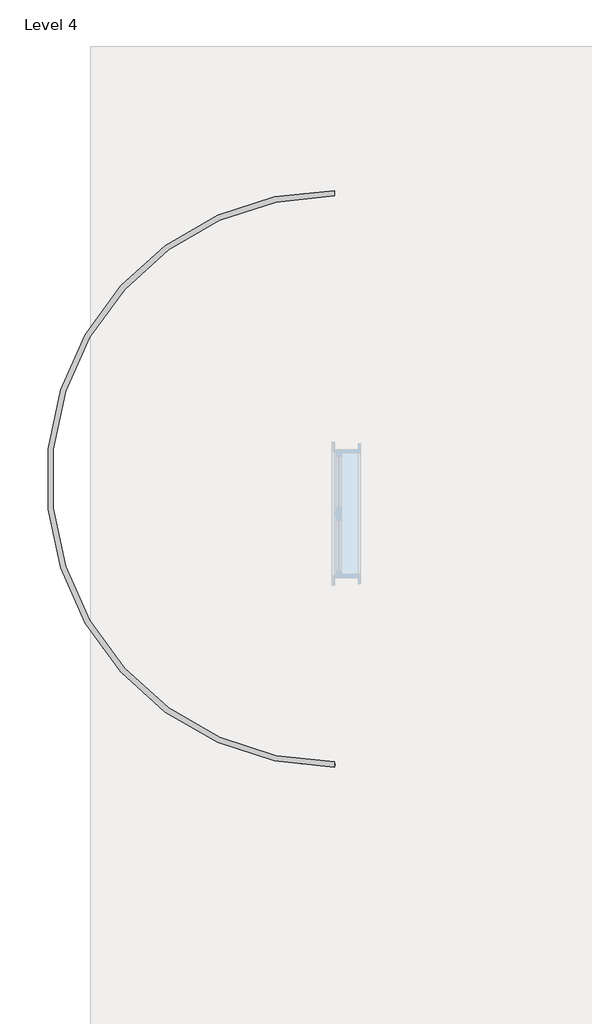
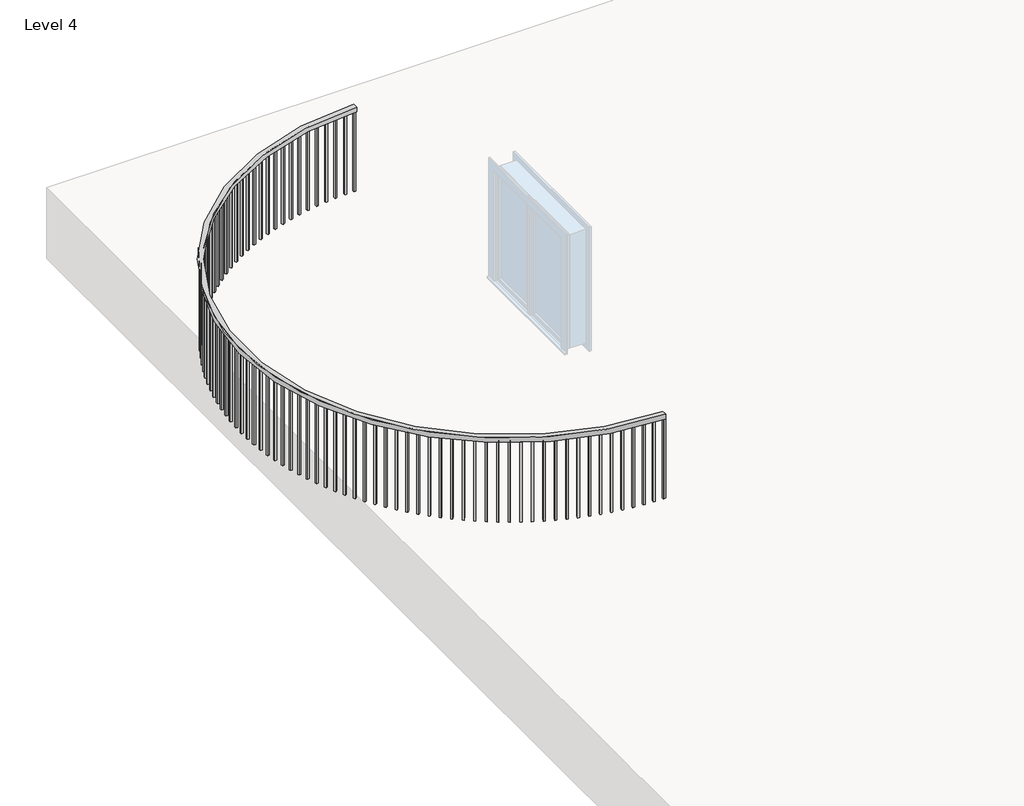
# One storey, part 2 of 2: 1 railing.
"""IFC4 building model written with IfcOpenShell, lengths in millimetres."""

from ifc_helpers import new_model, si_unit, point, frame, frame_2d, origin, place, context, project, spatial, polyline, circle_curve, trimmed, segment, composite_curve, outline, extrude, element, save

model = new_model("IFC4")

# Units and contexts
model_context = context("Model", 3, world=origin())
ifc_project = project(units=[si_unit("LENGTHUNIT", "METRE", prefix="MILLI")], contexts=[model_context])

# Site, building, storey
site = spatial("IfcSite", under=ifc_project)
building = spatial("IfcBuilding", under=site)
storey = spatial("IfcBuildingStorey", under=building, Name="Level 4", Elevation=9144.0)

# Railing
placement = place(None, origin())
element("IfcRailing", 1, ObjectType="Handrail - Rectangular", at=placement, inside=storey, context=model_context, shape_type="SweptSolid", body=[
    extrude(outline(composite_curve([segment(trimmed(circle_curve(frame_2d((-15728.6368919, 10326.9945075)), 2743.2), [point((-15728.6368919, 7583.7945075))], [point((-15728.6368919, 13070.1945075))], False, "CARTESIAN"), True, "CONTINUOUS"), segment(polyline([(-15728.6368919, 13070.1945075), (-15728.6368919, 13019.3945075)]), True, "CONTINUOUS"), segment(trimmed(circle_curve(frame_2d((-15728.6368919, 10326.9945075)), 2692.4), [point((-15728.6368919, 13019.3945075))], [point((-15728.6368919, 7634.5945075))], True, "CARTESIAN"), True, "CONTINUOUS"), segment(polyline([(-15728.6368919, 7634.5945075), (-15728.6368919, 7583.7945075)]), True, "CONTINUOUS")], self_intersect=False)), frame((0.0, 0.0, 10007.6), z_axis=(0.0, 0.0, 1.0), x_axis=(1.0, 0.0, 0.0)), (0.0, 0.0, 1.0), 50.8),
    extrude(outline(polyline([(-15741.9957848, 7599.6855919), (-15741.9690055, 7618.735573), (-15722.9190243, 7618.7087937), (-15722.9458036, 7599.6588126), (-15741.9957848, 7599.6855919)])), frame((0.0, 0.0, 9144.0), z_axis=(0.0, 0.0, 1.0), x_axis=(1.0, 0.0, 0.0)), (0.0, 0.0, 1.0), 863.6),
    extrude(outline(polyline([(-15843.9181793, 7602.0903613), (-15843.1794358, 7621.1260319), (-15824.1437651, 7620.3872884), (-15824.8825087, 7601.3516177), (-15843.9181793, 7602.0903613)])), frame((0.0, 0.0, 9144.0), z_axis=(0.0, 0.0, 1.0), x_axis=(1.0, 0.0, 0.0)), (0.0, 0.0, 1.0), 863.6),
    extrude(outline(polyline([(-15945.6794868, 7608.3027461), (-15944.2298113, 7627.297507), (-15925.2350504, 7625.8478315), (-15926.6847259, 7606.8530706), (-15945.6794868, 7608.3027461)])), frame((0.0, 0.0, 9144.0), z_axis=(0.0, 0.0, 1.0), x_axis=(1.0, 0.0, 0.0)), (0.0, 0.0, 1.0), 863.6),
    extrude(outline(polyline([(-16047.1375121, 7618.3140656), (-16044.9789303, 7637.2413746), (-16026.0516213, 7635.0827927), (-16028.2102032, 7616.1554838), (-16047.1375121, 7618.3140656)])), frame((0.0, 0.0, 9144.0), z_axis=(0.0, 0.0, 1.0), x_axis=(1.0, 0.0, 0.0)), (0.0, 0.0, 1.0), 863.6),
    extrude(outline(polyline([(-16148.150484, 7632.1103305), (-16145.2860122, 7650.9437397), (-16126.452603, 7648.0792678), (-16129.3170749, 7629.2458587), (-16148.150484, 7632.1103305)])), frame((0.0, 0.0, 9144.0), z_axis=(0.0, 0.0, 1.0), x_axis=(1.0, 0.0, 0.0)), (0.0, 0.0, 1.0), 863.6),
    extrude(outline(polyline([(-16248.5772532, 7649.6722628), (-16245.0108939, 7668.3854555), (-16226.2977012, 7664.8190963), (-16229.8640605, 7646.1059035), (-16248.5772532, 7649.6722628)])), frame((0.0, 0.0, 9144.0), z_axis=(0.0, 0.0, 1.0), x_axis=(1.0, 0.0, 0.0)), (0.0, 0.0, 1.0), 863.6),
    extrude(outline(polyline([(-16348.2774892, 7670.9753224), (-16344.014226, 7689.54215), (-16325.4473984, 7685.2788868), (-16329.7106616, 7666.7120592), (-16348.2774892, 7670.9753224)])), frame((0.0, 0.0, 9144.0), z_axis=(0.0, 0.0, 1.0), x_axis=(1.0, 0.0, 0.0)), (0.0, 0.0, 1.0), 863.6),
    extrude(outline(polyline([(-16447.1118772, 7695.9897418), (-16442.1576672, 7714.3842602), (-16423.7631489, 7709.4300502), (-16428.7173589, 7691.0355319), (-16447.1118772, 7695.9897418)])), frame((0.0, 0.0, 9144.0), z_axis=(0.0, 0.0, 1.0), x_axis=(1.0, 0.0, 0.0)), (0.0, 0.0, 1.0), 863.6),
    extrude(outline(polyline([(-16544.9423119, 7724.6805674), (-16539.3040779, 7742.8770731), (-16521.1075722, 7737.2388391), (-16526.7458062, 7719.0423334), (-16544.9423119, 7724.6805674)])), frame((0.0, 0.0, 9144.0), z_axis=(0.0, 0.0, 1.0), x_axis=(1.0, 0.0, 0.0)), (0.0, 0.0, 1.0), 863.6),
    extrude(outline(polyline([(-16641.632091, 7757.0077083), (-16635.3177115, 7774.9807746), (-16617.3446452, 7768.6663951), (-16623.6590247, 7750.6933288), (-16641.632091, 7757.0077083)])), frame((0.0, 0.0, 9144.0), z_axis=(0.0, 0.0, 1.0), x_axis=(1.0, 0.0, 0.0)), (0.0, 0.0, 1.0), 863.6),
    extrude(outline(polyline([(-16737.0461061, 7792.9259926), (-16730.0644044, 7810.6505051), (-16712.3398919, 7803.6688034), (-16719.3215936, 7785.9442909), (-16737.0461061, 7792.9259926)])), frame((0.0, 0.0, 9144.0), z_axis=(0.0, 0.0, 1.0), x_axis=(1.0, 0.0, 0.0)), (0.0, 0.0, 1.0), 863.6),
    extrude(outline(polyline([(-16831.0510314, 7832.3852302), (-16823.4117634, 7849.8364217), (-16805.9605719, 7842.1971536), (-16813.59984, 7824.7459621), (-16831.0510314, 7832.3852302)])), frame((0.0, 0.0, 9144.0), z_axis=(0.0, 0.0, 1.0), x_axis=(1.0, 0.0, 0.0)), (0.0, 0.0, 1.0), 863.6),
    extrude(outline(polyline([(-16923.5155103, 7875.3302832), (-16915.2293505, 7892.4837684), (-16898.0758652, 7884.1976086), (-16906.362025, 7867.0441234), (-16923.5155103, 7875.3302832)])), frame((0.0, 0.0, 9144.0), z_axis=(0.0, 0.0, 1.0), x_axis=(1.0, 0.0, 0.0)), (0.0, 0.0, 1.0), 863.6),
    extrude(outline(polyline([(-17014.3103383, 7921.7011427), (-17005.3888654, 7938.5329525), (-16988.5570556, 7929.6114796), (-16997.4785285, 7912.7796698), (-17014.3103383, 7921.7011427)])), frame((0.0, 0.0, 9144.0), z_axis=(0.0, 0.0, 1.0), x_axis=(1.0, 0.0, 0.0)), (0.0, 0.0, 1.0), 863.6),
    extrude(outline(polyline([(-17103.3086445, 7971.4330131), (-17093.7643247, 7987.9196276), (-17077.2777101, 7978.3753079), (-17086.8220299, 7961.8886933), (-17103.3086445, 7971.4330131)])), frame((0.0, 0.0, 9144.0), z_axis=(0.0, 0.0, 1.0), x_axis=(1.0, 0.0, 0.0)), (0.0, 0.0, 1.0), 863.6),
    extrude(outline(polyline([(-17190.3860679, 8024.4564019), (-17180.2322379, 8040.5747838), (-17164.1138559, 8030.4209539), (-17174.2676859, 8014.3025719), (-17190.3860679, 8024.4564019)])), frame((0.0, 0.0, 9144.0), z_axis=(0.0, 0.0, 1.0), x_axis=(1.0, 0.0, 0.0)), (0.0, 0.0, 1.0), 863.6),
    extrude(outline(polyline([(-17275.4209318, 8080.6972174), (-17264.67178, 8096.424844), (-17248.9441535, 8085.6756922), (-17259.6933053, 8069.9480657), (-17275.4209318, 8080.6972174)])), frame((0.0, 0.0, 9144.0), z_axis=(0.0, 0.0, 1.0), x_axis=(1.0, 0.0, 0.0)), (0.0, 0.0, 1.0), 863.6),
    extrude(outline(polyline([(-17358.2944137, 8140.0768723), (-17346.9649603, 8155.3917666), (-17331.6500661, 8144.0623132), (-17342.9795194, 8128.747419), (-17358.2944137, 8140.0768723)])), frame((0.0, 0.0, 9144.0), z_axis=(0.0, 0.0, 1.0), x_axis=(1.0, 0.0, 0.0)), (0.0, 0.0, 1.0), 863.6),
    extrude(outline(polyline([(-17438.8907113, 8202.512393), (-17426.9967874, 8217.3931549), (-17412.1160255, 8205.499231), (-17424.0099494, 8190.6184691), (-17438.8907113, 8202.512393)])), frame((0.0, 0.0, 9144.0), z_axis=(0.0, 0.0, 1.0), x_axis=(1.0, 0.0, 0.0)), (0.0, 0.0, 1.0), 863.6),
    extrude(outline(polyline([(-17517.0972041, 8267.9165359), (-17504.6554295, 8282.3423719), (-17490.2295935, 8269.9005973), (-17502.671368, 8255.4747613), (-17517.0972041, 8267.9165359)])), frame((0.0, 0.0, 9144.0), z_axis=(0.0, 0.0, 1.0), x_axis=(1.0, 0.0, 0.0)), (0.0, 0.0, 1.0), 863.6),
    extrude(outline(polyline([(-17592.8046111, 8336.1979092), (-17579.8323713, 8350.1486616), (-17565.8816189, 8337.1764217), (-17578.8538587, 8323.2256693), (-17592.8046111, 8336.1979092)])), frame((0.0, 0.0, 9144.0), z_axis=(0.0, 0.0, 1.0), x_axis=(1.0, 0.0, 0.0)), (0.0, 0.0, 1.0), 863.6),
    extrude(outline(polyline([(-17665.9071435, 8407.2611006), (-17652.422565, 8420.7172754), (-17638.9663901, 8407.2326969), (-17652.4509687, 8393.7765221), (-17665.9071435, 8407.2611006)])), frame((0.0, 0.0, 9144.0), z_axis=(0.0, 0.0, 1.0), x_axis=(1.0, 0.0, 0.0)), (0.0, 0.0, 1.0), 863.6),
    extrude(outline(polyline([(-17736.3026522, 8481.0068109), (-17722.3245775, 8493.9496053), (-17709.3817831, 8479.9715306), (-17723.3598578, 8467.0287361), (-17736.3026522, 8481.0068109)])), frame((0.0, 0.0, 9144.0), z_axis=(0.0, 0.0, 1.0), x_axis=(1.0, 0.0, 0.0)), (0.0, 0.0, 1.0), 863.6),
    extrude(outline(polyline([(-17803.8927708, 8557.3319921), (-17789.4407321, 8569.7433206), (-17777.0294035, 8555.2912819), (-17791.4814423, 8542.8799533), (-17803.8927708, 8557.3319921)])), frame((0.0, 0.0, 9144.0), z_axis=(0.0, 0.0, 1.0), x_axis=(1.0, 0.0, 0.0)), (0.0, 0.0, 1.0), 863.6),
    extrude(outline(polyline([(-17868.583053, 8636.1299922), (-17853.6772446, 8647.992512), (-17841.8147248, 8633.0867036), (-17856.7205331, 8621.2241838), (-17868.583053, 8636.1299922)])), frame((0.0, 0.0, 9144.0), z_axis=(0.0, 0.0, 1.0), x_axis=(1.0, 0.0, 0.0)), (0.0, 0.0, 1.0), 863.6),
    extrude(outline(polyline([(-17930.2831044, 8717.2907036), (-17914.9443548, 8728.5878387), (-17903.6472197, 8713.2490891), (-17918.9859693, 8701.951954), (-17930.2831044, 8717.2907036)])), frame((0.0, 0.0, 9144.0), z_axis=(0.0, 0.0, 1.0), x_axis=(1.0, 0.0, 0.0)), (0.0, 0.0, 1.0), 863.6),
    extrude(outline(polyline([(-17988.9067092, 8800.7007172), (-17973.1564519, 8811.4166817), (-17962.4404874, 8795.6664245), (-17978.1907447, 8784.9504599), (-17988.9067092, 8800.7007172)])), frame((0.0, 0.0, 9144.0), z_axis=(0.0, 0.0, 1.0), x_axis=(1.0, 0.0, 0.0)), (0.0, 0.0, 1.0), 863.6),
    extrude(outline(polyline([(-18044.3719504, 8886.2434811), (-18028.2321938, 8896.3633011), (-18018.1123738, 8880.2235446), (-18034.2521303, 8870.1037245), (-18044.3719504, 8886.2434811)])), frame((0.0, 0.0, 9144.0), z_axis=(0.0, 0.0, 1.0), x_axis=(1.0, 0.0, 0.0)), (0.0, 0.0, 1.0), 863.6),
    extrude(outline(polyline([(-18096.6013241, 8973.7994628), (-18080.094621, 8983.3089976), (-18070.5850862, 8966.8022945), (-18087.0917894, 8957.2927597), (-18096.6013241, 8973.7994628)])), frame((0.0, 0.0, 9144.0), z_axis=(0.0, 0.0, 1.0), x_axis=(1.0, 0.0, 0.0)), (0.0, 0.0, 1.0), 863.6),
    extrude(outline(polyline([(-18145.5218483, 9063.2463171), (-18128.6712641, 9072.1322785), (-18119.7853026, 9055.2816943), (-18136.6358868, 9046.3957328), (-18145.5218483, 9063.2463171)])), frame((0.0, 0.0, 9144.0), z_axis=(0.0, 0.0, 1.0), x_axis=(1.0, 0.0, 0.0)), (0.0, 0.0, 1.0), 863.6),
    extrude(outline(polyline([(-18191.0651643, 9154.4590562), (-18173.894245, 9162.7090277), (-18165.6442735, 9145.5381083), (-18182.8151929, 9137.2881369), (-18191.0651643, 9154.4590562)])), frame((0.0, 0.0, 9144.0), z_axis=(0.0, 0.0, 1.0), x_axis=(1.0, 0.0, 0.0)), (0.0, 0.0, 1.0), 863.6),
    extrude(outline(polyline([(-18233.1676328, 9247.3102252), (-18215.7003719, 9254.9126786), (-18208.0979185, 9237.4454177), (-18225.5651793, 9229.8429643), (-18233.1676328, 9247.3102252)])), frame((0.0, 0.0, 9144.0), z_axis=(0.0, 0.0, 1.0), x_axis=(1.0, 0.0, 0.0)), (0.0, 0.0, 1.0), 863.6),
    extrude(outline(polyline([(-18271.7704221, 9341.6700793), (-18254.0312274, 9348.6143915), (-18247.0869153, 9330.8751968), (-18264.82611, 9323.9308846), (-18271.7704221, 9341.6700793)])), frame((0.0, 0.0, 9144.0), z_axis=(0.0, 0.0, 1.0), x_axis=(1.0, 0.0, 0.0)), (0.0, 0.0, 1.0), 863.6),
    extrude(outline(polyline([(-18306.8195913, 9437.4067659), (-18288.8332504, 9443.6832333), (-18282.5567831, 9425.6968925), (-18300.5431239, 9419.4204251), (-18306.8195913, 9437.4067659)])), frame((0.0, 0.0, 9144.0), z_axis=(0.0, 0.0, 1.0), x_axis=(1.0, 0.0, 0.0)), (0.0, 0.0, 1.0), 863.6),
    extrude(outline(polyline([(-18338.2661646, 9534.3865084), (-18320.0578106, 9539.9863606), (-18314.4579584, 9521.7780066), (-18332.6663124, 9516.1781544), (-18338.2661646, 9534.3865084)])), frame((0.0, 0.0, 9144.0), z_axis=(0.0, 0.0, 1.0), x_axis=(1.0, 0.0, 0.0)), (0.0, 0.0, 1.0), 863.6),
    extrude(outline(polyline([(-18366.0662006, 9632.4737931), (-18347.6612768, 9637.3892053), (-18342.7458646, 9618.9842814), (-18361.1507885, 9614.0688692), (-18366.0662006, 9632.4737931)])), frame((0.0, 0.0, 9144.0), z_axis=(0.0, 0.0, 1.0), x_axis=(1.0, 0.0, 0.0)), (0.0, 0.0, 1.0), 863.6),
    extrude(outline(polyline([(-18390.1808532, 9731.5315588), (-18371.6050774, 9735.7556625), (-18367.3809737, 9717.1798866), (-18385.9567496, 9712.955783), (-18390.1808532, 9731.5315588)])), frame((0.0, 0.0, 9144.0), z_axis=(0.0, 0.0, 1.0), x_axis=(1.0, 0.0, 0.0)), (0.0, 0.0, 1.0), 863.6),
    extrude(outline(polyline([(-18410.576426, 9831.4213883), (-18391.8557549, 9834.9482809), (-18388.3288623, 9816.2276097), (-18407.0495335, 9812.7007171), (-18410.576426, 9831.4213883)])), frame((0.0, 0.0, 9144.0), z_axis=(0.0, 0.0, 1.0), x_axis=(1.0, 0.0, 0.0)), (0.0, 0.0, 1.0), 863.6),
    extrude(outline(polyline([(-18427.2244196, 9932.0037015), (-18408.3850122, 9934.8284548), (-18405.560259, 9915.9890475), (-18424.3996663, 9913.1642942), (-18427.2244196, 9932.0037015)])), frame((0.0, 0.0, 9144.0), z_axis=(0.0, 0.0, 1.0), x_axis=(1.0, 0.0, 0.0)), (0.0, 0.0, 1.0), 863.6),
    extrude(outline(polyline([(-18440.1015709, 10033.1379509), (-18421.1697524, 10035.2566177), (-18419.0510856, 10016.3247992), (-18437.9829041, 10014.2061324), (-18440.1015709, 10033.1379509)])), frame((0.0, 0.0, 9144.0), z_axis=(0.0, 0.0, 1.0), x_axis=(1.0, 0.0, 0.0)), (0.0, 0.0, 1.0), 863.6),
    extrude(outline(polyline([(-18449.1898863, 10134.6828176), (-18430.1921108, 10136.0924374), (-18428.782491, 10117.094662), (-18447.7802664, 10115.6850421), (-18449.1898863, 10134.6828176)])), frame((0.0, 0.0, 9144.0), z_axis=(0.0, 0.0, 1.0), x_axis=(1.0, 0.0, 0.0)), (0.0, 0.0, 1.0), 863.6),
    extrude(outline(polyline([(-18454.4766663, 10236.4964089), (-18435.4394802, 10237.1950121), (-18434.740877, 10218.157826), (-18453.7780631, 10217.4592228), (-18454.4766663, 10236.4964089)])), frame((0.0, 0.0, 9144.0), z_axis=(0.0, 0.0, 1.0), x_axis=(1.0, 0.0, 0.0)), (0.0, 0.0, 1.0), 863.6),
    extrude(outline(polyline([(-18455.9545234, 10338.4364568), (-18436.9045281, 10338.4230671), (-18436.9179178, 10319.3730718), (-18455.967913, 10319.3864615), (-18455.9545234, 10338.4364568)])), frame((0.0, 0.0, 9144.0), z_axis=(0.0, 0.0, 1.0), x_axis=(1.0, 0.0, 0.0)), (0.0, 0.0, 1.0), 863.6),
    extrude(outline(polyline([(-18453.6213926, 10440.3605163), (-18434.5852074, 10439.6351526), (-18435.3105712, 10420.5989673), (-18454.3467564, 10421.3243311), (-18453.6213926, 10440.3605163)])), frame((0.0, 0.0, 9144.0), z_axis=(0.0, 0.0, 1.0), x_axis=(1.0, 0.0, 0.0)), (0.0, 0.0, 1.0), 863.6),
    extrude(outline(polyline([(-18447.4805342, 10542.1261652), (-18428.4847591, 10540.6898408), (-18429.9210834, 10521.6940657), (-18448.9168585, 10523.13039), (-18447.4805342, 10542.1261652)])), frame((0.0, 0.0, 9144.0), z_axis=(0.0, 0.0, 1.0), x_axis=(1.0, 0.0, 0.0)), (0.0, 0.0, 1.0), 863.6),
    extrude(outline(polyline([(-18437.5405288, 10643.5912021), (-18418.6117074, 10641.4459242), (-18420.7569852, 10622.5171027), (-18439.6858067, 10624.6623806), (-18437.5405288, 10643.5912021)])), frame((0.0, 0.0, 9144.0), z_axis=(0.0, 0.0, 1.0), x_axis=(1.0, 0.0, 0.0)), (0.0, 0.0, 1.0), 863.6),
    extrude(outline(polyline([(-18423.8152662, 10744.613846), (-18404.9798483, 10741.7626123), (-18407.8310821, 10722.9271944), (-18426.6664999, 10725.7784281), (-18423.8152662, 10744.613846)])), frame((0.0, 0.0, 9144.0), z_axis=(0.0, 0.0, 1.0), x_axis=(1.0, 0.0, 0.0)), (0.0, 0.0, 1.0), 863.6),
    extrude(outline(polyline([(-18406.3239251, 10845.0529341), (-18387.6082304, 10841.4997286), (-18391.1614358, 10822.7840338), (-18409.8771306, 10826.3372393), (-18406.3239251, 10845.0529341)])), frame((0.0, 0.0, 9144.0), z_axis=(0.0, 0.0, 1.0), x_axis=(1.0, 0.0, 0.0)), (0.0, 0.0, 1.0), 863.6),
    extrude(outline(polyline([(-18385.0909469, 10944.7681188), (-18366.5211274, 10940.5179066), (-18370.7713395, 10921.9480871), (-18389.341159, 10926.1982992), (-18385.0909469, 10944.7681188)])), frame((0.0, 0.0, 9144.0), z_axis=(0.0, 0.0, 1.0), x_axis=(1.0, 0.0, 0.0)), (0.0, 0.0, 1.0), 863.6),
    extrude(outline(polyline([(-18360.1460013, 11043.6200641), (-18341.7480054, 11038.6787843), (-18346.6892852, 11020.2807884), (-18365.0872811, 11025.2220682), (-18360.1460013, 11043.6200641)])), frame((0.0, 0.0, 9144.0), z_axis=(0.0, 0.0, 1.0), x_axis=(1.0, 0.0, 0.0)), (0.0, 0.0, 1.0), 863.6),
    extrude(outline(polyline([(-18331.5239448, 11141.4706405), (-18313.3234807, 11135.8451977), (-18318.9489235, 11117.6447336), (-18337.1493876, 11123.2701765), (-18331.5239448, 11141.4706405)])), frame((0.0, 0.0, 9144.0), z_axis=(0.0, 0.0, 1.0), x_axis=(1.0, 0.0, 0.0)), (0.0, 0.0, 1.0), 863.6),
    extrude(outline(polyline([(-18299.2647721, 11238.1831175), (-18281.287272, 11231.8813723), (-18287.5890173, 11213.9038722), (-18305.5665173, 11220.2056175), (-18299.2647721, 11238.1831175)])), frame((0.0, 0.0, 9144.0), z_axis=(0.0, 0.0, 1.0), x_axis=(1.0, 0.0, 0.0)), (0.0, 0.0, 1.0), 863.6),
    extrude(outline(polyline([(-18263.4135602, 11333.6223549), (-18245.6841449, 11326.6531129), (-18252.6533869, 11308.9236976), (-18270.3828021, 11315.8929396), (-18263.4135602, 11333.6223549)])), frame((0.0, 0.0, 9144.0), z_axis=(0.0, 0.0, 1.0), x_axis=(1.0, 0.0, 0.0)), (0.0, 0.0, 1.0), 863.6),
    extrude(outline(polyline([(-18224.0204055, 11427.6549917), (-18206.5638489, 11420.0279914), (-18214.1908492, 11402.5714348), (-18231.6474057, 11410.1984351), (-18224.0204055, 11427.6549917)])), frame((0.0, 0.0, 9144.0), z_axis=(0.0, 0.0, 1.0), x_axis=(1.0, 0.0, 0.0)), (0.0, 0.0, 1.0), 863.6),
    extrude(outline(polyline([(-18181.1403535, 11520.1496324), (-18163.9810484, 11511.8755313), (-18172.2551495, 11494.7162262), (-18189.4144546, 11502.9903273), (-18181.1403535, 11520.1496324)])), frame((0.0, 0.0, 9144.0), z_axis=(0.0, 0.0, 1.0), x_axis=(1.0, 0.0, 0.0)), (0.0, 0.0, 1.0), 863.6),
    extrude(outline(polyline([(-18134.8333222, 11610.9770307), (-18117.995246, 11602.0673905), (-18126.9048862, 11585.2293142), (-18143.7429624, 11594.1389544), (-18134.8333222, 11610.9770307)])), frame((0.0, 0.0, 9144.0), z_axis=(0.0, 0.0, 1.0), x_axis=(1.0, 0.0, 0.0)), (0.0, 0.0, 1.0), 863.6),
    extrude(outline(polyline([(-18085.1640183, 11700.0102698), (-18068.6706994, 11690.4775403), (-18078.2034289, 11673.9842214), (-18094.6967478, 11683.5169509), (-18085.1640183, 11700.0102698)])), frame((0.0, 0.0, 9144.0), z_axis=(0.0, 0.0, 1.0), x_axis=(1.0, 0.0, 0.0)), (0.0, 0.0, 1.0), 863.6),
    extrude(outline(polyline([(-18032.2018467, 11787.1249402), (-18016.0763318, 11776.9824419), (-18026.2188302, 11760.8569271), (-18042.344345, 11770.9994254), (-18032.2018467, 11787.1249402)])), frame((0.0, 0.0, 9144.0), z_axis=(0.0, 0.0, 1.0), x_axis=(1.0, 0.0, 0.0)), (0.0, 0.0, 1.0), 863.6),
    extrude(outline(polyline([(-17976.0208133, 11872.199313), (-17960.2856354, 11861.4612184), (-17971.0237301, 11845.7260405), (-17986.758908, 11856.4641351), (-17976.0208133, 11872.199313)])), frame((0.0, 0.0, 9144.0), z_axis=(0.0, 0.0, 1.0), x_axis=(1.0, 0.0, 0.0)), (0.0, 0.0, 1.0), 863.6),
    extrude(outline(polyline([(-17916.6994223, 11955.1145106), (-17901.3765687, 11943.7958244), (-17912.6952549, 11928.4729708), (-17928.0181085, 11939.791657), (-17916.6994223, 11955.1145106)])), frame((0.0, 0.0, 9144.0), z_axis=(0.0, 0.0, 1.0), x_axis=(1.0, 0.0, 0.0)), (0.0, 0.0, 1.0), 863.6),
    extrude(outline(polyline([(-17854.3205656, 12035.7546722), (-17839.4314475, 12023.8712105), (-17851.3149093, 12008.9820924), (-17866.2040274, 12020.8655541), (-17854.3205656, 12035.7546722)])), frame((0.0, 0.0, 9144.0), z_axis=(0.0, 0.0, 1.0), x_axis=(1.0, 0.0, 0.0)), (0.0, 0.0, 1.0), 863.6),
    extrude(outline(polyline([(-17788.9714078, 12114.0071162), (-17774.5368304, 12101.5754842), (-17786.9684624, 12087.1409068), (-17801.4030399, 12099.5725388), (-17788.9714078, 12114.0071162)])), frame((0.0, 0.0, 9144.0), z_axis=(0.0, 0.0, 1.0), x_axis=(1.0, 0.0, 0.0)), (0.0, 0.0, 1.0), 863.6),
    extrude(outline(polyline([(-17720.7432638, 12189.7624974), (-17706.783397, 12176.8000663), (-17719.7458282, 12162.8401996), (-17733.7056949, 12175.8026307), (-17720.7432638, 12189.7624974)])), frame((0.0, 0.0, 9144.0), z_axis=(0.0, 0.0, 1.0), x_axis=(1.0, 0.0, 0.0)), (0.0, 0.0, 1.0), 863.6),
    extrude(outline(polyline([(-17649.7314714, 12262.9149599), (-17636.265822, 12249.4398426), (-17649.7409393, 12235.9741932), (-17663.2065887, 12249.4493105), (-17649.7314714, 12262.9149599)])), frame((0.0, 0.0, 9144.0), z_axis=(0.0, 0.0, 1.0), x_axis=(1.0, 0.0, 0.0)), (0.0, 0.0, 1.0), 863.6),
    extrude(outline(polyline([(-17576.0352582, 12333.3622847), (-17563.0826422, 12319.3933106), (-17577.0516164, 12306.4406946), (-17590.0042323, 12320.4096688), (-17576.0352582, 12333.3622847)])), frame((0.0, 0.0, 9144.0), z_axis=(0.0, 0.0, 1.0), x_axis=(1.0, 0.0, 0.0)), (0.0, 0.0, 1.0), 863.6),
    extrude(outline(polyline([(-17499.7576028, 12401.0060332), (-17487.3361194, 12386.5627216), (-17501.779431, 12374.1412382), (-17514.2009144, 12388.5845499), (-17499.7576028, 12401.0060332)])), frame((0.0, 0.0, 9144.0), z_axis=(0.0, 0.0, 1.0), x_axis=(1.0, 0.0, 0.0)), (0.0, 0.0, 1.0), 863.6),
    extrude(outline(polyline([(-17421.0050909, 12465.751684), (-17409.1320972, 12450.8542171), (-17424.0295641, 12438.9812234), (-17435.9025578, 12453.8786903), (-17421.0050909, 12465.751684)])), frame((0.0, 0.0, 9144.0), z_axis=(0.0, 0.0, 1.0), x_axis=(1.0, 0.0, 0.0)), (0.0, 0.0, 1.0), 863.6),
    extrude(outline(polyline([(-17339.8877666, 12527.5087656), (-17328.5798531, 12512.1779602), (-17343.9106585, 12500.8700467), (-17355.218572, 12516.2008521), (-17339.8877666, 12527.5087656)])), frame((0.0, 0.0, 9144.0), z_axis=(0.0, 0.0, 1.0), x_axis=(1.0, 0.0, 0.0)), (0.0, 0.0, 1.0), 863.6),
    extrude(outline(polyline([(-17256.5189783, 12586.1909822), (-17245.791946, 12570.4482607), (-17261.5346675, 12559.7212285), (-17272.2616997, 12575.46395), (-17256.5189783, 12586.1909822)])), frame((0.0, 0.0, 9144.0), z_axis=(0.0, 0.0, 1.0), x_axis=(1.0, 0.0, 0.0)), (0.0, 0.0, 1.0), 863.6),
    extrude(outline(polyline([(-17171.0152203, 12641.716335), (-17160.8840587, 12625.5836953), (-17177.0166983, 12615.4525337), (-17187.14786, 12631.5851733), (-17171.0152203, 12641.716335)])), frame((0.0, 0.0, 9144.0), z_axis=(0.0, 0.0, 1.0), x_axis=(1.0, 0.0, 0.0)), (0.0, 0.0, 1.0), 863.6),
    extrude(outline(polyline([(-17083.4959706, 12694.0072362), (-17073.9748361, 12677.5072211), (-17090.4748512, 12667.9860867), (-17099.9959857, 12684.4861018), (-17083.4959706, 12694.0072362)])), frame((0.0, 0.0, 9144.0), z_axis=(0.0, 0.0, 1.0), x_axis=(1.0, 0.0, 0.0)), (0.0, 0.0, 1.0), 863.6),
    extrude(outline(polyline([(-16994.0835232, 12742.9906177), (-16985.1857201, 12726.1462833), (-17002.0300546, 12717.2484803), (-17010.9278576, 12734.0928147), (-16994.0835232, 12742.9906177)])), frame((0.0, 0.0, 9144.0), z_axis=(0.0, 0.0, 1.0), x_axis=(1.0, 0.0, 0.0)), (0.0, 0.0, 1.0), 863.6),
    extrude(outline(polyline([(-16902.9028175, 12788.5980331), (-16894.6407792, 12771.4329166), (-16911.8058957, 12763.1708783), (-16920.067934, 12780.3359948), (-16902.9028175, 12788.5980331)])), frame((0.0, 0.0, 9144.0), z_axis=(0.0, 0.0, 1.0), x_axis=(1.0, 0.0, 0.0)), (0.0, 0.0, 1.0), 863.6),
    extrude(outline(polyline([(-16810.081264, 12830.7657533), (-16802.4665353, 12813.3038403), (-16819.9284483, 12805.6891115), (-16827.543177, 12823.1510246), (-16810.081264, 12830.7657533)])), frame((0.0, 0.0, 9144.0), z_axis=(0.0, 0.0, 1.0), x_axis=(1.0, 0.0, 0.0)), (0.0, 0.0, 1.0), 863.6),
    extrude(outline(polyline([(-16715.7485659, 12869.4348557), (-16708.7917871, 12851.7005464), (-16726.5260965, 12844.7437676), (-16733.4828752, 12862.4780769), (-16715.7485659, 12869.4348557)])), frame((0.0, 0.0, 9144.0), z_axis=(0.0, 0.0, 1.0), x_axis=(1.0, 0.0, 0.0)), (0.0, 0.0, 1.0), 863.6),
    extrude(outline(polyline([(-16620.0365379, 12904.5513065), (-16613.74743, 12886.5693817), (-16631.7293549, 12880.2802738), (-16638.0184627, 12898.2621987), (-16620.0365379, 12904.5513065)])), frame((0.0, 0.0, 9144.0), z_axis=(0.0, 0.0, 1.0), x_axis=(1.0, 0.0, 0.0)), (0.0, 0.0, 1.0), 863.6),
    extrude(outline(polyline([(-16523.0789222, 12936.0660362), (-16517.4662733, 12917.8616226), (-16535.6706868, 12912.2489737), (-16541.2833357, 12930.4533872), (-16523.0789222, 12936.0660362)])), frame((0.0, 0.0, 9144.0), z_axis=(0.0, 0.0, 1.0), x_axis=(1.0, 0.0, 0.0)), (0.0, 0.0, 1.0), 863.6),
    extrude(outline(polyline([(-16425.0112015, 12963.9350078), (-16420.0828543, 12945.5335433), (-16438.4843187, 12940.6051961), (-16443.4126659, 12959.0066606), (-16425.0112015, 12963.9350078)])), frame((0.0, 0.0, 9144.0), z_axis=(0.0, 0.0, 1.0), x_axis=(1.0, 0.0, 0.0)), (0.0, 0.0, 1.0), 863.6),
    extrude(outline(polyline([(-16325.9704097, 12988.119279), (-16321.7332507, 12969.5464768), (-16340.306053, 12965.3093178), (-16344.5432119, 12983.8821201), (-16325.9704097, 12988.119279)])), frame((0.0, 0.0, 9144.0), z_axis=(0.0, 0.0, 1.0), x_axis=(1.0, 0.0, 0.0)), (0.0, 0.0, 1.0), 863.6),
    extrude(outline(polyline([(-16226.0949403, 13008.5850563), (-16222.5548904, 12989.8668687), (-16241.273078, 12986.3268188), (-16244.8131279, 13005.0450064), (-16226.0949403, 13008.5850563)])), frame((0.0, 0.0, 9144.0), z_axis=(0.0, 0.0, 1.0), x_axis=(1.0, 0.0, 0.0)), (0.0, 0.0, 1.0), 863.6),
    extrude(outline(polyline([(-16125.5243533, 13025.3037418), (-16122.686359, 13006.4663246), (-16141.5237763, 13003.6283304), (-16144.3617705, 13022.4657476), (-16125.5243533, 13025.3037418)])), frame((0.0, 0.0, 9144.0), z_axis=(0.0, 0.0, 1.0), x_axis=(1.0, 0.0, 0.0)), (0.0, 0.0, 1.0), 863.6),
    extrude(outline(polyline([(-16024.3991798, 13038.2519741), (-16022.2672069, 13019.3216494), (-16041.1975316, 13017.1896766), (-16043.3295045, 13036.1200012), (-16024.3991798, 13038.2519741)])), frame((0.0, 0.0, 9144.0), z_axis=(0.0, 0.0, 1.0), x_axis=(1.0, 0.0, 0.0)), (0.0, 0.0, 1.0), 863.6),
    extrude(outline(polyline([(-15922.8607261, 13047.41166), (-15921.4377537, 13028.41488), (-15940.4345336, 13026.9919075), (-15941.8575061, 13045.9886875), (-15922.8607261, 13047.41166)])), frame((0.0, 0.0, 9144.0), z_axis=(0.0, 0.0, 1.0), x_axis=(1.0, 0.0, 0.0)), (0.0, 0.0, 1.0), 863.6),
    extrude(outline(polyline([(-15821.0508759, 13052.7700002), (-15820.3388922, 13033.7333099), (-15839.3755825, 13033.0213262), (-15840.0875662, 13052.0580165), (-15821.0508759, 13052.7700002)])), frame((0.0, 0.0, 9144.0), z_axis=(0.0, 0.0, 1.0), x_axis=(1.0, 0.0, 0.0)), (0.0, 0.0, 1.0), 863.6),
    extrude(outline(polyline([(-15747.7201959, 7599.7196389), (-15747.653432, 7618.7695219), (-15728.603549, 7618.702758), (-15728.6703128, 7599.652875), (-15747.7201959, 7599.7196389)])), frame((0.0, 0.0, 9144.0), z_axis=(0.0, 0.0, 1.0), x_axis=(1.0, 0.0, 0.0)), (0.0, 0.0, 1.0), 863.6),
    extrude(outline(polyline([(-15728.6703128, 13054.3361399), (-15728.603549, 13035.2862569), (-15747.653432, 13035.219493), (-15747.7201959, 13054.2693761), (-15728.6703128, 13054.3361399)])), frame((0.0, 0.0, 9144.0), z_axis=(0.0, 0.0, 1.0), x_axis=(1.0, 0.0, 0.0)), (0.0, 0.0, 1.0), 863.6),
])

save(model, "model.ifc")

# Revit data of these elements
# Type "Handrail - Rectangular"
#   Assembly Code = "C2010400"
#   built-in parameter 1008612 = 0.0416667 (stored number, unit not read)
#   built-in parameter 1008611 = 0.0416667 (stored number, unit not read)
#   built-in parameter 1008609 = 0.333333 (stored number, unit not read)
#   built-in parameter 1008604 = 0.166667 (stored number, unit not read)
#   built-in parameter 1008603 = 0.166667 (stored number, unit not read)
#   Railing Height = 3' - 0"
#   built-in parameter 1008630 = 2
#   built-in parameter 1008610 = 2
#   built-in parameter 1008618 = Baluster - Square : 3/4"
# Element 1 (IfcRailing, "Handrail - Rectangular")
#   Phase Created = New Construction
